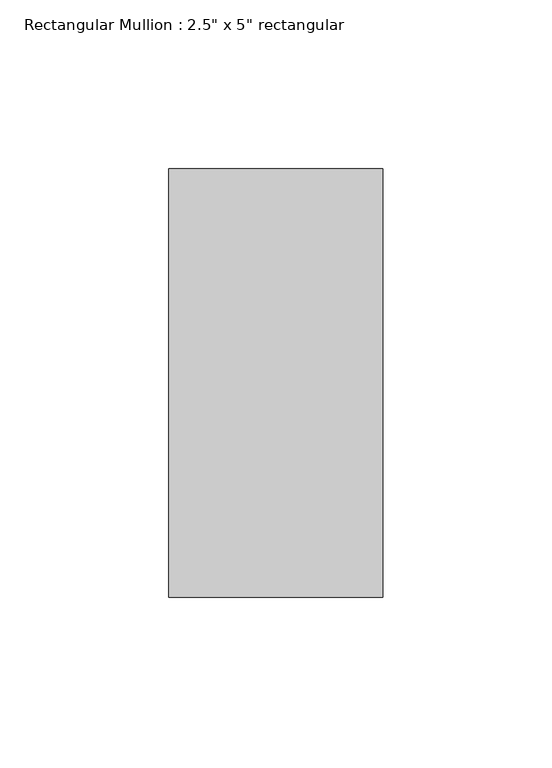
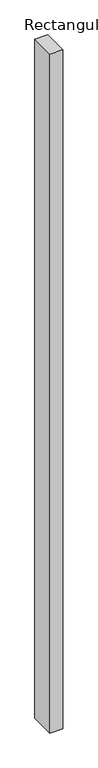
"""IFC4 building model written with IfcOpenShell, lengths in millimetres: member geometry."""

from ifc_helpers import new_model, si_unit, frame, origin, place, context, project, spatial, polyline, outline, extrude, source, transform, mapped, element, save


def member_eb03db27(model_context):
    return source(origin(), model_context, "Body", "SweptSolid", [
        extrude(outline(polyline([(0.0, 63.5), (0.0, -63.5), (-63.5, -63.5), (-63.5, 63.5), (0.0, 63.5)])), frame((0.0, 0.0, -3498.5550856), z_axis=(0.0, 0.0, 1.0), x_axis=(1.0, 0.0, 0.0)), (0.0, 0.0, 1.0), 3498.5550856),
    ])


if __name__ == "__main__":
    model = new_model("IFC4")
    model_context = context("Model", 3, world=origin())
    ifc_project = project(units=[si_unit("LENGTHUNIT", "METRE", prefix="MILLI")], contexts=[model_context])
    site = spatial("IfcSite", under=ifc_project)
    building = spatial("IfcBuilding", under=site)
    placement = place(None, origin())
    member_shape = member_eb03db27(model_context)
    element("IfcMember", 1, ObjectType="Rectangular Mullion : 2.5\" x 5\" rectangular", at=placement, inside=building, context=model_context, shape_type="MappedRepresentation", body=[
        mapped(member_shape, transform((0.0, 0.0, 0.0), x_axis=(1.0, 0.0, 0.0), y_axis=(0.0, 1.0, 0.0), z_axis=(0.0, 0.0, 1.0))),
    ])
    save(model, "model.ifc")

# Revit data of these elements
# Type "Rectangular Mullion : 2.5\" x 5\" rectangular"
#   built-in parameter 1007304 = 0.416667 (stored number, unit not read)
#   built-in parameter 1007301 = 0.104167 (stored number, unit not read)
#   built-in parameter 1007300 = 0.104167 (stored number, unit not read)
# Element 1 (IfcMember, "Rectangular Mullion : 2.5\" x 5\" rectangular")
#   Materials on its faces: "Iron, Ductile"
# Materials
#   "Iron, Ductile": class "Metal", colour RGB 0 0 0, transparency 0, Description = "Ductile cast iron", Cost = 0
